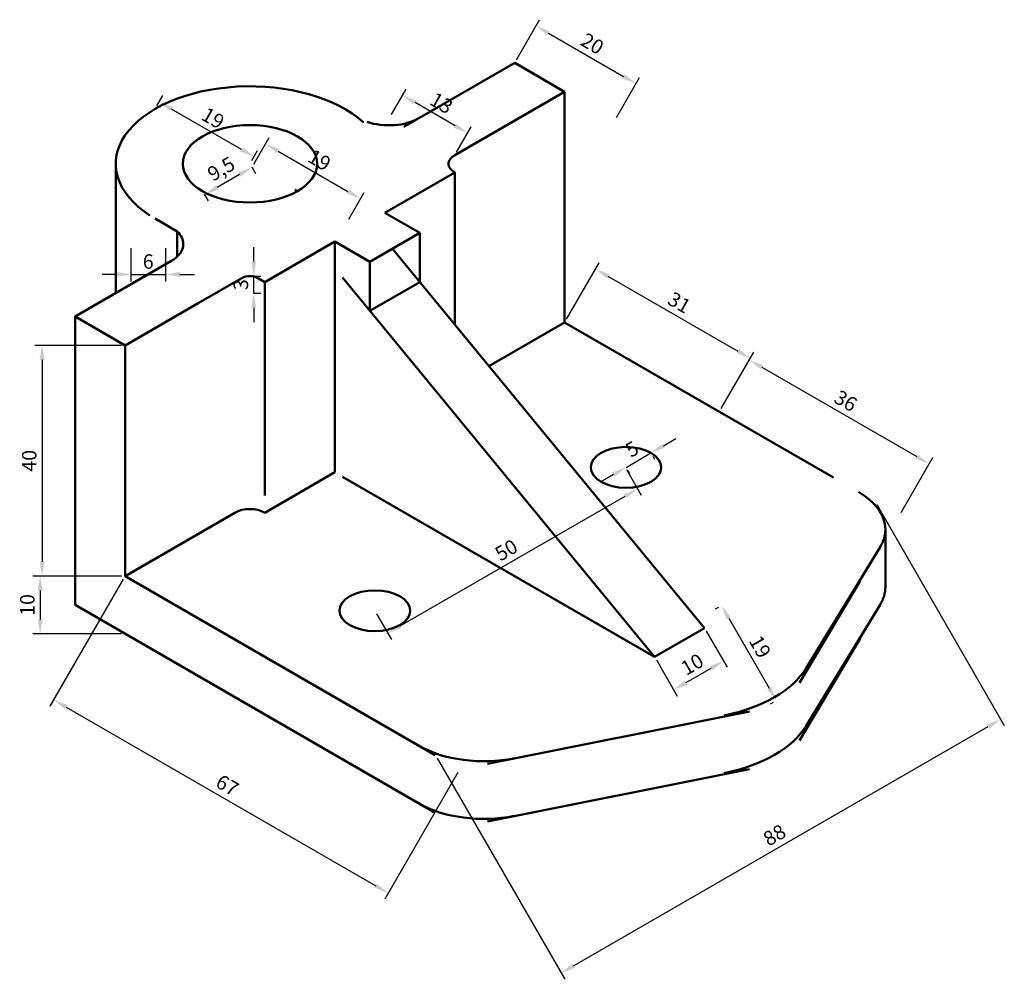
# Model space of a CAD drawing. Units: millimetres. Extents: x 1310 to 1481, y 167 to 333.
import ezdxf

# ---------------------------------------------------------------- set-up
doc = ezdxf.new("R2010")
doc.units = ezdxf.units.MM
doc.layers.add('M-DIMS', color=2, linetype='Continuous', lineweight=25)
doc.layers.add('M-OUTL', color=7, linetype='Continuous', lineweight=50)
doc.styles.get("Standard").update_dxf_attribs({"font": 'arial.ttf'})
doc.dimstyles.new('ISO-25', dxfattribs={"dimtxt": 2.5, "dimasz": 2.5, "dimexe": 1.25, "dimexo": 0.625, "dimtad": 1, "dimtxsty": 'Standard', "dimcen": 2.5, "dimadec": 0, "dimazin": 0, "dimtfac": 1, "dimtmove": 0, "dimatfit": 3, "dimfxl": 1, "dimarcsym": 0})

# ---------------------------------------------------------------- blocks, each defined once
blk = doc.blocks.new('*D1')
at = {"layer": 'Defpoints', "color": 0, "transparency": 16777216}
for p in [(1429.12, 227.54), (1420.46, 222.54), (1432.42, 221.82)]:
    blk.add_point(p, dxfattribs=at)
at = {"layer": 'M-DIMS', "color": 0, "lineweight": -2, "transparency": 16777216}
for p, q in [((1429.43, 227), (1433.05, 220.74)), ((1420.77, 222), (1424.39, 215.74)), ((1425.93, 218.07), (1430.26, 220.57))]:
    blk.add_line(p, q, dxfattribs=at)
at = {"layer": 'M-DIMS', "color": 0, "transparency": 16777216}
for points in [[(1430.05, 220.93), (1430.46, 220.21), (1432.42, 221.82)], [(1425.72, 218.43), (1426.13, 217.71), (1423.76, 216.82)]]:
    blk.add_solid(points, dxfattribs=at)
at = {"layer": 'M-DIMS', "color": 0, "transparency": 16777216, "insert": (1427.14, 220.97), "char_height": 2.5, "attachment_point": 5, "rotation": 30}
blk.add_mtext('10', dxfattribs=at)
blk = doc.blocks.new('*D2')
at = {"layer": 'Defpoints', "color": 0, "transparency": 16777216}
for p in [(1432.08, 231.41), (1441.57, 214.96), (1441.58, 214.96)]:
    blk.add_point(p, dxfattribs=at)
at = {"layer": 'M-DIMS', "color": 0, "lineweight": -2, "transparency": 16777216}
for p, q in [((1431.54, 231.1), (1430.99, 230.79)), ((1433.32, 229.25), (1440.32, 217.12)), ((1441.04, 214.65), (1440.49, 214.33))]:
    blk.add_line(p, q, dxfattribs=at)
at = {"layer": 'M-DIMS', "color": 0, "transparency": 16777216}
for points in [[(1433.68, 229.45), (1432.96, 229.04), (1432.07, 231.41)], [(1440.68, 217.33), (1439.96, 216.91), (1441.57, 214.96)]]:
    blk.add_solid(points, dxfattribs=at)
at = {"layer": 'M-DIMS', "color": 0, "transparency": 16777216, "insert": (1438.47, 224.14), "char_height": 2.5, "attachment_point": 5, "rotation": 300}
blk.add_mtext('19', dxfattribs=at)
blk = doc.blocks.new('*D3')
at = {"layer": 'Defpoints', "color": 0, "transparency": 16777216}
for p in [(1415.26, 255.54), (1417.51, 251.65), (1371.96, 230.54)]:
    blk.add_point(p, dxfattribs=at)
at = {"layer": 'M-DIMS', "color": 0, "lineweight": -2, "transparency": 16777216}
for p, q in [((1415.57, 255), (1418.13, 250.56)), ((1376.37, 227.9), (1415.34, 250.4)), ((1372.27, 230), (1374.83, 225.56))]:
    blk.add_line(p, q, dxfattribs=at)
at = {"layer": 'M-DIMS', "color": 0, "transparency": 16777216}
for points in [[(1415.14, 250.76), (1415.55, 250.04), (1417.51, 251.65)], [(1376.16, 228.26), (1376.58, 227.54), (1374.21, 226.65)]]:
    blk.add_solid(points, dxfattribs=at)
at = {"layer": 'M-DIMS', "color": 0, "transparency": 16777216, "insert": (1394.91, 240.79), "char_height": 2.5, "attachment_point": 5, "rotation": 30}
blk.add_mtext('50', dxfattribs=at)
blk = doc.blocks.new('*D4')
at = {"layer": 'Defpoints', "color": 0, "transparency": 16777216}
for p in [(1404.87, 280.54), (1437.06, 274.3), (1431.72, 265.04)]:
    blk.add_point(p, dxfattribs=at)
at = {"layer": 'M-DIMS', "color": 0, "lineweight": -2, "transparency": 16777216}
for p, q in [((1405.18, 281.08), (1410.84, 290.88)), ((1412.38, 288.55), (1434.9, 275.55)), ((1432.03, 265.58), (1437.69, 275.38))]:
    blk.add_line(p, q, dxfattribs=at)
at = {"layer": 'M-DIMS', "color": 0, "transparency": 16777216}
for points in [[(1412.59, 288.91), (1412.17, 288.19), (1410.22, 289.8)], [(1435.11, 275.91), (1434.69, 275.19), (1437.06, 274.3)]]:
    blk.add_solid(points, dxfattribs=at)
at = {"layer": 'M-DIMS', "color": 0, "transparency": 16777216, "insert": (1424.59, 283.7), "char_height": 2.5, "attachment_point": 5, "rotation": 330}
blk.add_mtext('31', dxfattribs=at)
blk = doc.blocks.new('*D5')
at = {"layer": 'Defpoints', "color": 0, "transparency": 16777216}
for p in [(1431.72, 265.04), (1468.08, 256.02), (1462.89, 247.04)]:
    blk.add_point(p, dxfattribs=at)
at = {"layer": 'M-DIMS', "color": 0, "lineweight": -2, "transparency": 16777216}
for p, q in [((1432.03, 265.58), (1437.52, 275.1)), ((1439.06, 272.77), (1465.91, 257.27)), ((1463.21, 247.58), (1468.7, 257.1))]:
    blk.add_line(p, q, dxfattribs=at)
at = {"layer": 'M-DIMS', "color": 0, "transparency": 16777216}
for points in [[(1439.27, 273.13), (1438.85, 272.4), (1436.9, 274.02)], [(1466.12, 257.63), (1465.7, 256.9), (1468.08, 256.02)]]:
    blk.add_solid(points, dxfattribs=at)
at = {"layer": 'M-DIMS', "color": 0, "transparency": 16777216, "insert": (1453.44, 266.66), "char_height": 2.5, "attachment_point": 5, "rotation": 330}
blk.add_mtext('36', dxfattribs=at)
blk = doc.blocks.new('*D6')
at = {"layer": 'Defpoints', "color": 0, "transparency": 16777216}
for p in [(1458.65, 249.49), (1480.46, 211.71), (1382.44, 205.49)]:
    blk.add_point(p, dxfattribs=at)
at = {"layer": 'M-DIMS', "color": 0, "lineweight": -2, "transparency": 16777216}
for p, q in [((1458.97, 248.95), (1481.09, 210.63)), ((1406.42, 168.96), (1478.3, 210.46)), ((1382.76, 204.95), (1404.88, 166.63))]:
    blk.add_line(p, q, dxfattribs=at)
at = {"layer": 'M-DIMS', "color": 0, "transparency": 16777216}
for points in [[(1478.09, 210.82), (1478.51, 210.1), (1480.46, 211.71)], [(1406.21, 169.32), (1406.63, 168.6), (1404.25, 167.71)]]:
    blk.add_solid(points, dxfattribs=at)
at = {"layer": 'M-DIMS', "color": 0, "transparency": 16777216, "insert": (1441.41, 191.36), "char_height": 2.5, "attachment_point": 5, "rotation": 30}
blk.add_mtext('88', dxfattribs=at)
blk = doc.blocks.new('*D7')
at = {"layer": 'Defpoints', "color": 0, "transparency": 16777216}
for p in [(1328.66, 236.54), (1386.68, 203.04), (1374.3, 181.59)]:
    blk.add_point(p, dxfattribs=at)
at = {"layer": 'M-DIMS', "color": 0, "lineweight": -2, "transparency": 16777216}
for p, q in [((1328.35, 236), (1315.65, 214.01)), ((1318.44, 213.84), (1372.13, 182.84)), ((1386.37, 202.5), (1373.67, 180.51))]:
    blk.add_line(p, q, dxfattribs=at)
at = {"layer": 'M-DIMS', "color": 0, "transparency": 16777216}
for points in [[(1318.65, 214.2), (1318.23, 213.48), (1316.27, 215.09)], [(1372.34, 183.2), (1371.92, 182.48), (1374.3, 181.59)]]:
    blk.add_solid(points, dxfattribs=at)
at = {"layer": 'M-DIMS', "color": 0, "transparency": 16777216, "insert": (1346.24, 199.99), "char_height": 2.5, "attachment_point": 5, "rotation": 330}
blk.add_mtext('67', dxfattribs=at)
blk = doc.blocks.new('*D8')
at = {"layer": 'Defpoints', "color": 0, "transparency": 16777216}
for p in [(1328.66, 236.54), (1313.94, 226.54), (1328.66, 226.54)]:
    blk.add_point(p, dxfattribs=at)
at = {"layer": 'M-DIMS', "color": 0, "lineweight": -2, "transparency": 16777216}
for p, q in [((1328.03, 236.54), (1312.69, 236.54)), ((1313.94, 234.04), (1313.94, 229.04)), ((1328.03, 226.54), (1312.69, 226.54))]:
    blk.add_line(p, q, dxfattribs=at)
at = {"layer": 'M-DIMS', "color": 0, "transparency": 16777216}
for points in [[(1313.52, 234.04), (1314.36, 234.04), (1313.94, 236.54)], [(1313.52, 229.04), (1314.36, 229.04), (1313.94, 226.54)]]:
    blk.add_solid(points, dxfattribs=at)
at = {"layer": 'M-DIMS', "color": 0, "transparency": 16777216, "insert": (1312.04, 231.54), "char_height": 2.5, "attachment_point": 5, "rotation": 90}
blk.add_mtext('10', dxfattribs=at)
blk = doc.blocks.new('*D9')
at = {"layer": 'Defpoints', "color": 0, "transparency": 16777216}
for p in [(1350.31, 308.04), (1342.08, 303.29), (1342.44, 302.67)]:
    blk.add_point(p, dxfattribs=at)
at = {"layer": 'M-DIMS', "color": 0, "lineweight": -2, "transparency": 16777216}
for p, q in [((1350.62, 307.5), (1351.29, 306.34)), ((1348.5, 306.17), (1344.61, 303.92)), ((1342.39, 302.75), (1343.07, 301.59))]:
    blk.add_line(p, q, dxfattribs=at)
at = {"layer": 'M-DIMS', "color": 0, "transparency": 16777216}
for points in [[(1348.29, 306.53), (1348.71, 305.81), (1350.67, 307.42)], [(1344.4, 304.28), (1344.81, 303.56), (1342.44, 302.67)]]:
    blk.add_solid(points, dxfattribs=at)
at = {"layer": 'M-DIMS', "color": 0, "transparency": 16777216, "insert": (1345.49, 306.89), "char_height": 2.5, "attachment_point": 5, "rotation": 30}
blk.add_mtext('9,5', dxfattribs=at)
blk = doc.blocks.new('*D10')
at = {"layer": 'Defpoints', "color": 0, "transparency": 16777216}
for p in [(1333.86, 317.54), (1334.57, 318.78), (1350.31, 308.04)]:
    blk.add_point(p, dxfattribs=at)
at = {"layer": 'M-DIMS', "color": 0, "lineweight": -2, "transparency": 16777216}
for p, q in [((1334.17, 318.08), (1335.2, 319.86)), ((1348.86, 310.53), (1336.74, 317.53)), ((1350.62, 308.58), (1351.65, 310.36))]:
    blk.add_line(p, q, dxfattribs=at)
at = {"layer": 'M-DIMS', "color": 0, "transparency": 16777216}
for points in [[(1336.94, 317.89), (1336.53, 317.17), (1334.57, 318.78)], [(1349.07, 310.89), (1348.65, 310.17), (1351.03, 309.28)]]:
    blk.add_solid(points, dxfattribs=at)
at = {"layer": 'M-DIMS', "color": 0, "transparency": 16777216, "insert": (1343.75, 315.68), "char_height": 2.5, "attachment_point": 5, "rotation": 330}
blk.add_mtext('19', dxfattribs=at)
blk = doc.blocks.new('*D11')
at = {"layer": 'Defpoints', "color": 0, "transparency": 16777216}
for p in [(1376.78, 319.89), (1374.56, 316.04), (1385.82, 309.54)]:
    blk.add_point(p, dxfattribs=at)
at = {"layer": 'M-DIMS', "color": 0, "lineweight": -2, "transparency": 16777216}
for p, q in [((1374.87, 316.58), (1377.41, 320.97)), ((1385.87, 314.64), (1378.95, 318.64)), ((1386.13, 310.08), (1388.66, 314.47))]:
    blk.add_line(p, q, dxfattribs=at)
at = {"layer": 'M-DIMS', "color": 0, "transparency": 16777216}
for points in [[(1379.15, 319), (1378.74, 318.28), (1376.78, 319.89)], [(1386.08, 315), (1385.66, 314.28), (1388.04, 313.39)]]:
    blk.add_solid(points, dxfattribs=at)
at = {"layer": 'M-DIMS', "color": 0, "transparency": 16777216, "insert": (1383.36, 318.29), "char_height": 2.5, "attachment_point": 5, "rotation": 330}
blk.add_mtext('13', dxfattribs=at)
blk = doc.blocks.new('*D12')
at = {"layer": 'Defpoints', "color": 0, "transparency": 16777216}
for p in [(1329.68, 294.06), (1335.68, 294.06), (1335.68, 288.86)]:
    blk.add_point(p, dxfattribs=at)
at = {"layer": 'M-DIMS', "color": 0, "lineweight": -2, "transparency": 16777216}
for p, q in [((1329.68, 293.43), (1329.68, 287.61)), ((1335.68, 293.43), (1335.68, 287.61)), ((1327.18, 288.86), (1324.68, 288.86)), ((1329.68, 288.86), (1335.68, 288.86)), ((1338.18, 288.86), (1340.68, 288.86))]:
    blk.add_line(p, q, dxfattribs=at)
at = {"layer": 'M-DIMS', "color": 0, "transparency": 16777216}
for points in [[(1327.18, 289.28), (1327.18, 288.45), (1329.68, 288.86)], [(1338.18, 289.28), (1338.18, 288.45), (1335.68, 288.86)]]:
    blk.add_solid(points, dxfattribs=at)
at = {"layer": 'M-DIMS', "color": 0, "transparency": 16777216, "insert": (1332.68, 290.76), "char_height": 2.5, "attachment_point": 5}
blk.add_mtext('6', dxfattribs=at)
blk = doc.blocks.new('*D13')
at = {"layer": 'Defpoints', "color": 0, "transparency": 16777216}
for p in [(1350.31, 288.58), (1350.97, 288.58), (1350.31, 285.58)]:
    blk.add_point(p, dxfattribs=at)
at = {"layer": 'M-DIMS', "color": 0, "lineweight": -2, "transparency": 16777216}
for p, q in [((1350.97, 291.08), (1350.97, 293.58)), ((1350.93, 288.58), (1352.22, 288.58)), ((1350.97, 285.58), (1350.97, 288.58)), ((1350.93, 285.58), (1352.22, 285.58)), ((1350.97, 283.08), (1350.97, 280.58))]:
    blk.add_line(p, q, dxfattribs=at)
at = {"layer": 'M-DIMS', "color": 0, "transparency": 16777216}
for points in [[(1350.56, 291.08), (1351.39, 291.08), (1350.97, 288.58)], [(1350.56, 283.08), (1351.39, 283.08), (1350.97, 285.58)]]:
    blk.add_solid(points, dxfattribs=at)
at = {"layer": 'M-DIMS', "color": 0, "transparency": 16777216, "insert": (1349.07, 287.08), "char_height": 2.5, "attachment_point": 5, "rotation": 90}
blk.add_mtext('3', dxfattribs=at)
blk = doc.blocks.new('*D14')
at = {"layer": 'Defpoints', "color": 0, "transparency": 16777216}
for p in [(1396.21, 325.54), (1417.23, 321.94), (1413.53, 315.54)]:
    blk.add_point(p, dxfattribs=at)
at = {"layer": 'M-DIMS', "color": 0, "lineweight": -2, "transparency": 16777216}
for p, q in [((1396.52, 326.08), (1400.53, 333.02)), ((1402.07, 330.69), (1415.06, 323.19)), ((1413.84, 316.08), (1417.85, 323.02))]:
    blk.add_line(p, q, dxfattribs=at)
at = {"layer": 'M-DIMS', "color": 0, "transparency": 16777216}
for points in [[(1402.28, 331.05), (1401.86, 330.33), (1399.91, 331.94)], [(1415.27, 323.55), (1414.85, 322.83), (1417.23, 321.94)]]:
    blk.add_solid(points, dxfattribs=at)
at = {"layer": 'M-DIMS', "color": 0, "transparency": 16777216, "insert": (1409.52, 328.59), "char_height": 2.5, "attachment_point": 5, "rotation": 330}
blk.add_mtext('20', dxfattribs=at)
blk = doc.blocks.new('*D15')
at = {"layer": 'Defpoints', "color": 0, "transparency": 16777216}
for p in [(1328.66, 276.54), (1314.28, 236.54), (1328.66, 236.54)]:
    blk.add_point(p, dxfattribs=at)
at = {"layer": 'M-DIMS', "color": 0, "lineweight": -2, "transparency": 16777216}
for p, q in [((1328.03, 276.54), (1313.03, 276.54)), ((1314.28, 274.04), (1314.28, 239.04)), ((1328.03, 236.54), (1313.03, 236.54))]:
    blk.add_line(p, q, dxfattribs=at)
at = {"layer": 'M-DIMS', "color": 0, "transparency": 16777216}
for points in [[(1313.86, 274.04), (1314.7, 274.04), (1314.28, 276.54)], [(1313.86, 239.04), (1314.7, 239.04), (1314.28, 236.54)]]:
    blk.add_solid(points, dxfattribs=at)
at = {"layer": 'M-DIMS', "color": 0, "transparency": 16777216, "insert": (1312.38, 256.54), "char_height": 2.5, "attachment_point": 5, "rotation": 90}
blk.add_mtext('40', dxfattribs=at)
blk = doc.blocks.new('*D16')
at = {"layer": 'Defpoints', "color": 0, "transparency": 16777216}
for p in [(1419.84, 257.9), (1419.84, 257.9), (1415.51, 255.4)]:
    blk.add_point(p, dxfattribs=at)
at = {"layer": 'M-DIMS', "color": 0, "lineweight": -2, "transparency": 16777216}
for p, q in [((1422, 259.15), (1424.17, 260.4)), ((1415.51, 255.4), (1419.84, 257.9)), ((1420.15, 257.36), (1420.46, 256.82)), ((1415.82, 254.86), (1416.13, 254.32)), ((1413.34, 254.15), (1411.18, 252.9))]:
    blk.add_line(p, q, dxfattribs=at)
at = {"layer": 'M-DIMS', "color": 0, "transparency": 16777216}
for points in [[(1421.79, 259.51), (1422.21, 258.79), (1419.84, 257.9)], [(1413.13, 254.51), (1413.55, 253.79), (1415.51, 255.4)]]:
    blk.add_solid(points, dxfattribs=at)
at = {"layer": 'M-DIMS', "color": 0, "transparency": 16777216, "insert": (1416.72, 258.29), "char_height": 2.5, "attachment_point": 5, "rotation": 30}
blk.add_mtext('5', dxfattribs=at)
blk = doc.blocks.new('*D17')
at = {"layer": 'Defpoints', "color": 0, "transparency": 16777216}
for p in [(1350.67, 307.42), (1369.48, 302), (1367.12, 297.92)]:
    blk.add_point(p, dxfattribs=at)
at = {"layer": 'M-DIMS', "color": 0, "lineweight": -2, "transparency": 16777216}
for p, q in [((1350.98, 307.96), (1353.65, 312.58)), ((1355.19, 310.25), (1367.31, 303.25)), ((1367.43, 298.46), (1370.1, 303.08))]:
    blk.add_line(p, q, dxfattribs=at)
at = {"layer": 'M-DIMS', "color": 0, "transparency": 16777216}
for points in [[(1355.4, 310.61), (1354.98, 309.89), (1353.02, 311.5)], [(1367.52, 303.61), (1367.1, 302.89), (1369.48, 302)]]:
    blk.add_solid(points, dxfattribs=at)
at = {"layer": 'M-DIMS', "color": 0, "transparency": 16777216, "insert": (1362.2, 308.4), "char_height": 2.5, "attachment_point": 5, "rotation": 330}
blk.add_mtext('19', dxfattribs=at)

msp = doc.modelspace()

# ---------------------------------------------------------------- linework, layer by layer
at = {"layer": 'M-OUTL'}
for p, q in [((1377.018, 314.46), (1396.209, 325.54)), ((1404.869, 320.54), (1396.209, 325.54)), ((1396.209, 325.54), (1404.869, 320.54)), ((1404.869, 320.54), (1385.817, 309.54)), ((1404.869, 320.54), (1404.869, 280.54)), ((1327.039, 308.04), (1327.039, 289.479)), ((1373.693, 299.54), (1385.817, 306.54)), ((1385.817, 306.54), (1385.817, 280.151)), ((1358.104, 303.54), (1358.537, 303.29)), ((1379.755, 296.04), (1373.693, 299.54)), ((1337.718, 296.31), (1333.855, 298.54)), ((1337.718, 296.31), (1337.718, 291.951)), ((1371.095, 291.04), (1379.755, 296.04)), ((1379.755, 287.518), (1379.755, 296.04)), ((1352.908, 287.54), (1365.032, 294.54)), ((1371.095, 291.04), (1365.032, 294.54)), ((1365.032, 294.54), (1365.032, 254.54)), ((1375, 293.294), (1429.118, 227.54)), ((1319.999, 281.54), (1336.61, 291.13)), ((1371.095, 282.518), (1371.095, 291.04)), ((1319.999, 281.54), (1332.684, 288.863)), ((1327.039, 289.479), (1327.039, 285.605)), ((1341.312, 283.845), (1348.81, 288.174)), ((1352.908, 287.54), (1351.81, 288.174)), ((1352.908, 287.54), (1352.908, 250.54)), ((1366.339, 288.294), (1420.458, 222.54)), ((1371.095, 282.518), (1379.755, 287.518)), ((1341.312, 283.845), (1328.659, 276.54)), ((1319.999, 231.54), (1319.999, 281.54)), ((1319.999, 281.54), (1328.659, 276.54)), ((1404.869, 280.54), (1391.737, 272.958)), ((1404.869, 280.54), (1431.716, 265.04)), ((1328.659, 276.54), (1328.659, 236.54)), ((1431.716, 265.04), (1451.467, 253.636)), ((1365.032, 254.54), (1352.908, 247.54)), ((1366.339, 253.785), (1420.458, 222.54)), ((1328.659, 236.54), (1347.712, 247.54)), ((1460.465, 234.635), (1460.465, 244.635)), ((1446.735, 220.574), (1459.559, 241.579)), ((1328.659, 236.54), (1382.444, 205.487)), ((1456.128, 235.712), (1445.572, 218.04)), ((1382.444, 195.487), (1319.999, 231.54)), ((1446.735, 210.574), (1459.559, 231.579)), ((1424.788, 225.04), (1429.118, 227.54)), ((1424.788, 225.04), (1429.118, 227.54)), ((1456.128, 225.712), (1445.572, 208.04)), ((1424.788, 225.04), (1420.458, 222.54)), ((1424.788, 225.04), (1420.458, 222.54)), ((1391.483, 203.995), (1436.912, 213.04)), ((1382.444, 205.487), (1382.444, 205.487)), ((1391.483, 193.995), (1436.912, 203.04))]:
    msp.add_line(p, q, dxfattribs=at)
msp.add_arc((1350.31, 285.575), 3, 60, 120, dxfattribs=at)
for centre, major_axis, start_param, end_param in [((1350.31, 308.04), (-23.27, 0), 3.7057582, 7.011559), ((1374.402, 318.95), (-7.349, 0), 1.0313598, 2.3561127), ((1388.415, 308.04), (3.674, 0), 2.3561949, 3.1415927), ((1388.415, 308.04), (3.674, 0), 3.1415927, 3.9269904), ((1331.413, 294.13), (7.349, 0), 0, 0.5394365), ((1331.413, 294.13), (7.349, 0), 5.4978689, 6.2831853), ((1444.543, 244.635), (-15.922, 0), 3.1415927, 3.9269908), ((1350.31, 246.04), (-3.674, 0), 3.9269912, 5.4977868), ((1444.543, 244.635), (-15.922, 0), 2.8027021, 3.1415927), ((1444.543, 234.635), (-15.922, 0), 2.8027021, 3.1415927), ((1424.788, 225.04), (23.27, 0), 5.0512791, 5.9442952), ((1424.788, 215.04), (23.27, 0), 5.0512791, 5.9442952), ((1390.849, 213.635), (15.922, 0), 3.9269908, 5.0512795), ((1390.849, 203.635), (15.922, 0), 3.9269908, 5.0512795)]:
    msp.add_ellipse(centre, major_axis=major_axis, ratio=0.5773503, start_param=start_param, end_param=end_param, dxfattribs=at)
for centre, major_axis in [((1350.31, 308.04), (-11.635, 0)), ((1415.505, 255.399), (-6.124, 0)), ((1371.96, 230.54), (-6.124, 0))]:
    msp.add_ellipse(centre, major_axis=major_axis, ratio=0.5773503, dxfattribs=at)

# ---------------------------------------------------------------- dimensions: what is measured, and where the dimension line sits
at = {"layer": 'M-DIMS'}
for p1, p2, distance, picture, middle in [((1396.209, 325.54), (1413.529, 315.54), 7.393, '*D14', (1409.517, 328.589)), ((1385.817, 309.54), (1374.558, 316.04), -4.443, '*D11', (1383.36, 318.285)), ((1350.31, 308.04), (1333.855, 317.54), -1.433, '*D10', (1343.75, 315.677)), ((1350.668, 307.419), (1367.122, 297.919), 4.712, '*D17', (1362.201, 308.397)), ((1350.31, 308.04), (1342.082, 303.29), 0.716, '*D9', (1345.49, 306.887)), ((1404.869, 280.54), (1431.716, 265.04), 10.695, '*D4', (1424.591, 283.699)), ((1431.716, 265.04), (1462.893, 247.04), 10.364, '*D5', (1453.438, 266.663)), ((1415.505, 255.399), (1419.836, 257.899), 0, '*D16', (1416.722, 258.291)), ((1371.96, 230.54), (1415.261, 255.54), -4.495, '*D3', (1394.908, 240.793)), ((1382.444, 205.487), (1458.654, 249.487), -43.62, '*D6', (1441.409, 191.357)), ((1328.659, 236.54), (1386.683, 203.04), -24.769, '*D7', (1346.237, 199.986)), ((1432.077, 231.414), (1441.577, 214.96), -0.005, '*D2', (1438.47, 224.135)), ((1420.458, 222.54), (1429.118, 227.54), -6.606, '*D1', (1427.14, 220.965))]:
    dim = msp.add_aligned_dim(p1=p1, p2=p2, distance=distance, dimstyle='ISO-25', override={"dimclrd": 0, "dimclre": 0, "dimclrt": 0}, dxfattribs=at)
    dim.commit()
    dim.dimension.update_dxf_attribs({"geometry": picture, "text_midpoint": middle})
dim = msp.add_linear_dim(base=(1335.684, 288.863), p1=(1329.684, 294.059), p2=(1335.684, 294.059), dimstyle='ISO-25', override={"dimclrd": 0, "dimclre": 0, "dimclrt": 0}, dxfattribs=at)
dim.commit()
dim.dimension.update_dxf_attribs({"geometry": '*D12', "text_midpoint": (1332.684, 290.765)})
for base, p1, p2, picture, middle in [((1350.974, 288.575), (1350.31, 285.575), (1350.31, 288.575), '*D13', (1349.072, 287.075)), ((1314.281, 236.54), (1328.659, 276.54), (1328.659, 236.54), '*D15', (1312.38, 256.54)), ((1313.939, 226.54), (1328.659, 236.54), (1328.659, 226.54), '*D8', (1312.038, 231.54))]:
    dim = msp.add_linear_dim(base=base, p1=p1, p2=p2, angle=90, dimstyle='ISO-25', override={"dimclrd": 0, "dimclre": 0, "dimclrt": 0}, dxfattribs=at)
    dim.commit()
    dim.dimension.update_dxf_attribs({"geometry": picture, "text_midpoint": middle})

doc.saveas('drawing.dxf')
